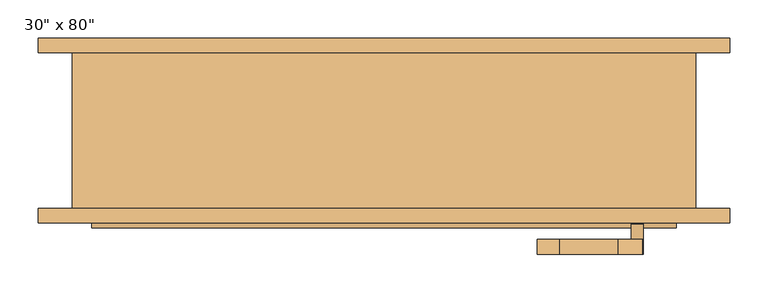
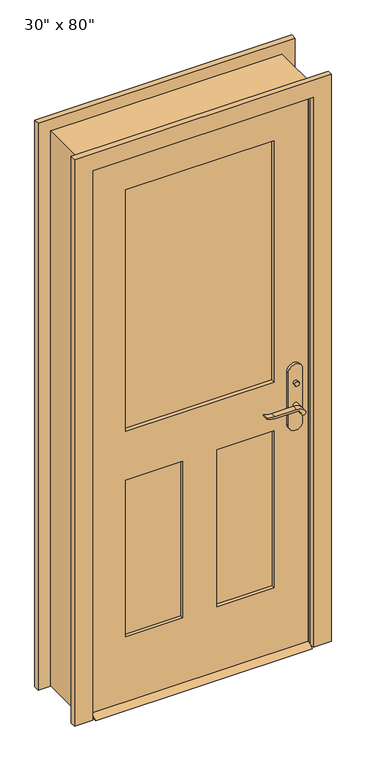
"""IFC4 building model written with IfcOpenShell, lengths in millimetres: door geometry."""

from ifc_helpers import new_model, si_unit, point, frame, frame_2d, origin, place, context, project, spatial, polyline, circle_curve, trimmed, segment, composite_curve, outline, extrude, faceted_brep, source, transform, mapped, element, save


def door_7e6851c9(model_context):
    return source(origin(), model_context, "Body", "SolidModel", [
        extrude(outline(polyline([(-63.5, 12.7), (-38.1, 0.0), (-123.825, 0.0), (-98.425, 12.7), (-63.5, 12.7)])), frame((-381.0, 0.0, 0.0), z_axis=(1.0, 0.0, 0.0), x_axis=(0.0, 1.0, 0.0)), (0.0, 0.0, 1.0), 762.0),
        extrude(outline(polyline([(335.2, -43.5), (335.2, -53.5), (325.2, -53.5), (325.2, -43.5), (335.2, -43.5)])), frame((0.0, 0.0, 981.9), z_axis=(0.0, 0.0, 1.0), x_axis=(1.0, 0.0, 0.0)), (0.0, 0.0, 1.0), 30.0),
        extrude(outline(composite_curve([segment(trimmed(circle_curve(frame_2d((996.9, 330.2)), 8.0), [point((996.9, 322.2))], [point((996.9, 338.2))], False, "CARTESIAN"), True, "CONTINUOUS"), segment(trimmed(circle_curve(frame_2d((996.9, 330.2)), 8.0), [point((996.9, 338.2))], [point((996.9, 322.2))], False, "CARTESIAN"), True, "CONTINUOUS")], self_intersect=False)), frame((0.0, -118.425, 0.0), z_axis=(0.0, 1.0, 0.0), x_axis=(0.0, 0.0, 1.0)), (0.0, 0.0, 1.0), 10.0),
        extrude(outline(composite_curve([segment(trimmed(circle_curve(frame_2d((897.1555521, 306.5324871)), 37.2832219), [point((919.0523287, 336.7081363))], [point((934.4, 304.8325667))], False, "CARTESIAN"), True, "CONTINUOUS"), segment(polyline([(934.4, 304.8325667), (934.4, 228.5564091)]), True, "CONTINUOUS"), segment(trimmed(circle_curve(frame_2d((1017.6850638, 228.6227909)), 83.2850902), [point((934.4, 228.5564091))], [point((939.4, 200.2))], True, "CARTESIAN"), True, "CONTINUOUS"), segment(polyline([(939.4, 200.2), (936.6135558, 200.2)]), True, "CONTINUOUS"), segment(trimmed(circle_curve(frame_2d((986.6709207, 232.1396612)), 59.3791355), [point((936.6135558, 200.2))], [point((927.4, 228.5564091))], False, "CARTESIAN"), True, "CONTINUOUS"), segment(polyline([(927.4, 228.5564091), (927.4, 304.8138099)]), True, "CONTINUOUS"), segment(trimmed(circle_curve(frame_2d((909.2738613, 304.8138099)), 18.1261387), [point((927.4, 304.8138099))], [point((914.4, 322.2))], True, "CARTESIAN"), True, "CONTINUOUS"), segment(trimmed(circle_curve(frame_2d((914.4, 330.2)), 8.0), [point((914.4, 322.2))], [point((919.0523287, 336.7081363))], False, "CARTESIAN"), True, "CONTINUOUS")], self_intersect=False)), frame((0.0, -23.5, 0.0), z_axis=(0.0, 1.0, 0.0), x_axis=(0.0, 0.0, 1.0)), (0.0, 0.0, 1.0), 20.0),
        extrude(outline(composite_curve([segment(trimmed(circle_curve(frame_2d((914.4, 330.2)), 8.0), [point((914.3999903, 322.2))], [point((919.0523287, 336.7081363))], False, "CARTESIAN"), True, "CONTINUOUS"), segment(trimmed(circle_curve(frame_2d((897.1555521, 306.5324871)), 37.2832219), [point((919.0523287, 336.7081363))], [point((934.4, 304.8325667))], False, "CARTESIAN"), True, "CONTINUOUS"), segment(polyline([(934.4, 304.8325667), (934.4, 228.5564091)]), True, "CONTINUOUS"), segment(trimmed(circle_curve(frame_2d((1017.6850638, 228.6227909)), 83.2850902), [point((934.4, 228.5564091))], [point((939.4, 200.2))], True, "CARTESIAN"), True, "CONTINUOUS"), segment(polyline([(939.4, 200.2), (936.6135558, 200.2)]), True, "CONTINUOUS"), segment(trimmed(circle_curve(frame_2d((986.6709207, 232.1396612)), 59.3791355), [point((936.6135558, 200.2))], [point((927.4, 228.5564091))], False, "CARTESIAN"), True, "CONTINUOUS"), segment(polyline([(927.4, 228.5564091), (927.4, 304.8138122)]), True, "CONTINUOUS"), segment(trimmed(circle_curve(frame_2d((909.2738682, 304.8138122)), 18.1261318), [point((927.4, 304.8138122))], [point((914.3999903, 322.2))], True, "CARTESIAN"), True, "CONTINUOUS")], self_intersect=False)), frame((0.0, -158.425, 0.0), z_axis=(0.0, 1.0, 0.0), x_axis=(0.0, 0.0, 1.0)), (0.0, 0.0, 1.0), 20.0),
        extrude(outline(composite_curve([segment(trimmed(circle_curve(frame_2d((914.4, 330.2)), 8.0), [point((914.4, 322.2))], [point((914.4, 338.2))], False, "CARTESIAN"), True, "CONTINUOUS"), segment(trimmed(circle_curve(frame_2d((914.4, 330.2)), 8.0), [point((914.4, 338.2))], [point((914.4, 322.2))], False, "CARTESIAN"), True, "CONTINUOUS")], self_intersect=False)), frame((0.0, -53.5, 0.0), z_axis=(0.0, 1.0, 0.0), x_axis=(0.0, 0.0, 1.0)), (0.0, 0.0, 1.0), 30.0),
        extrude(outline(composite_curve([segment(trimmed(circle_curve(frame_2d((914.4, 330.2)), 8.0), [point((914.4, 322.2))], [point((914.4, 338.2))], False, "CARTESIAN"), True, "CONTINUOUS"), segment(trimmed(circle_curve(frame_2d((914.4, 330.2)), 8.0), [point((914.4, 338.2))], [point((914.4, 322.2))], False, "CARTESIAN"), True, "CONTINUOUS")], self_intersect=False)), frame((0.0, -138.425, 0.0), z_axis=(0.0, 1.0, 0.0), x_axis=(0.0, 0.0, 1.0)), (0.0, 0.0, 1.0), 30.0),
        extrude(outline(composite_curve([segment(polyline([(844.4, 355.2), (1039.4, 355.2)]), True, "CONTINUOUS"), segment(trimmed(circle_curve(frame_2d((1039.4, 330.2)), 25.0), [point((1039.4, 355.2))], [point((1039.4, 305.2))], False, "CARTESIAN"), True, "CONTINUOUS"), segment(polyline([(1039.4, 305.2), (844.4, 305.2)]), True, "CONTINUOUS"), segment(trimmed(circle_curve(frame_2d((844.4, 330.2)), 25.0), [point((844.4, 305.2))], [point((844.4, 355.2))], False, "CARTESIAN"), True, "CONTINUOUS")], self_intersect=False)), frame((0.0, -63.5, 0.0), z_axis=(0.0, 1.0, 0.0), x_axis=(0.0, 0.0, 1.0)), (0.0, 0.0, 1.0), 10.0),
        extrude(outline(composite_curve([segment(polyline([(844.4, 355.2), (1039.4, 355.2)]), True, "CONTINUOUS"), segment(trimmed(circle_curve(frame_2d((1039.4, 330.2)), 25.0), [point((1039.4, 355.2))], [point((1039.4, 305.2))], False, "CARTESIAN"), True, "CONTINUOUS"), segment(polyline([(1039.4, 305.2), (844.4, 305.2)]), True, "CONTINUOUS"), segment(trimmed(circle_curve(frame_2d((844.4, 330.2)), 25.0), [point((844.4, 305.2))], [point((844.4, 355.2))], False, "CARTESIAN"), True, "CONTINUOUS")], self_intersect=False)), frame((0.0, -108.425, 0.0), z_axis=(0.0, 1.0, 0.0), x_axis=(0.0, 0.0, 1.0)), (0.0, 0.0, 1.0), 10.0),
        extrude(outline(polyline([(2032.0, -381.0), (12.7, -381.0), (12.7, 381.0), (2032.0, 381.0), (2032.0, -381.0)]), holes=[polyline([(1016.0, -260.35), (1911.35, -260.35), (1911.35, 260.35), (1016.0, 260.35), (1016.0, -260.35)]), polyline([(835.025, -60.325), (254.0, -60.325), (254.0, -260.35), (835.025, -260.35), (835.025, -60.325)]), polyline([(835.025, 260.35), (254.0, 260.35), (254.0, 60.325), (835.025, 60.325), (835.025, 260.35)])]), frame((0.0, -98.425, 0.0), z_axis=(0.0, 1.0, 0.0), x_axis=(0.0, 0.0, 1.0)), (0.0, 0.0, 1.0), 34.925),
        faceted_brep([(406.4, -98.425, 0.0), (381.0, -98.425, 0.0), (381.0, -63.5, 0.0), (368.3, -63.5, 0.0), (368.3, -28.575, 0.0), (381.0, -28.575, 0.0), (381.0, 104.775, 0.0), (406.4, 104.775, 0.0), (406.4, 104.775, 2057.4), (406.4, -98.425, 2057.4), (381.0, 104.775, 2032.0), (-381.0, 104.775, 2032.0), (-381.0, 104.775, 0.0), (-406.4, 104.775, 0.0), (-406.4, 104.775, 2057.4), (381.0, -28.575, 2032.0), (368.3, -28.575, 2019.3), (-368.3, -28.575, 2019.3), (-368.3, -28.575, 0.0), (-381.0, -28.575, 0.0), (-381.0, -28.575, 2032.0), (368.3, -63.5, 2019.3), (381.0, -63.5, 2032.0), (-381.0, -63.5, 2032.0), (-381.0, -63.5, 0.0), (-368.3, -63.5, 0.0), (-368.3, -63.5, 2019.3), (381.0, -98.425, 2032.0), (-406.4, -98.425, 2057.4), (-406.4, -98.425, 0.0), (-381.0, -98.425, 0.0), (-381.0, -98.425, 2032.0)], [[[0, 1, 2, 3, 4, 5, 6, 7]], [[7, 8, 9, 0]], [[6, 10, 11, 12, 13, 14, 8, 7]], [[5, 15, 10, 6]], [[4, 16, 17, 18, 19, 20, 15, 5]], [[3, 21, 16, 4]], [[2, 22, 23, 24, 25, 26, 21, 3]], [[1, 27, 22, 2]], [[0, 9, 28, 29, 30, 31, 27, 1]], [[8, 14, 28, 9]], [[15, 20, 11, 10]], [[21, 26, 17, 16]], [[27, 31, 23, 22]], [[29, 13, 12, 19, 18, 25, 24, 30]], [[14, 13, 29, 28]], [[20, 19, 12, 11]], [[26, 25, 18, 17]], [[31, 30, 24, 23]]]),
        extrude(outline(polyline([(-60.325, -75.1416667), (-60.325, -86.7833333), (-260.35, -86.7833333), (-260.35, -75.1416667), (-60.325, -75.1416667)])), frame((0.0, 0.0, 254.0), z_axis=(0.0, 0.0, 1.0), x_axis=(1.0, 0.0, 0.0)), (0.0, 0.0, 1.0), 581.025),
        extrude(outline(polyline([(260.35, -75.1416667), (260.35, -86.7833333), (60.325, -86.7833333), (60.325, -75.1416667), (260.35, -75.1416667)])), frame((0.0, 0.0, 254.0), z_axis=(0.0, 0.0, 1.0), x_axis=(1.0, 0.0, 0.0)), (0.0, 0.0, 1.0), 581.025),
        extrude(outline(polyline([(260.35, -77.47), (260.35, -84.455), (-260.35, -84.455), (-260.35, -77.47), (260.35, -77.47)])), frame((0.0, 0.0, 1016.0), z_axis=(0.0, 0.0, 1.0), x_axis=(1.0, 0.0, 0.0)), (0.0, 0.0, 1.0), 895.35),
        extrude(outline(polyline([(0.0, -387.35), (2038.35, -387.35), (2038.35, 387.35), (0.0, 387.35), (0.0, 450.85), (2101.85, 450.85), (2101.85, -450.85), (0.0, -450.85), (0.0, -387.35)])), frame((0.0, 104.775, 0.0), z_axis=(0.0, 1.0, 0.0), x_axis=(0.0, 0.0, 1.0)), (0.0, 0.0, 1.0), 19.05),
        extrude(outline(polyline([(0.0, -387.35), (2038.35, -387.35), (2038.35, 387.35), (0.0, 387.35), (0.0, 450.85), (2101.85, 450.85), (2101.85, -450.85), (0.0, -450.85), (0.0, -387.35)])), frame((0.0, -117.475, 0.0), z_axis=(0.0, 1.0, 0.0), x_axis=(0.0, 0.0, 1.0)), (0.0, 0.0, 1.0), 19.05),
    ])


if __name__ == "__main__":
    model = new_model("IFC4")
    model_context = context("Model", 3, world=origin())
    ifc_project = project(units=[si_unit("LENGTHUNIT", "METRE", prefix="MILLI")], contexts=[model_context])
    site = spatial("IfcSite", under=ifc_project)
    building = spatial("IfcBuilding", under=site)
    placement = place(None, origin())
    door_shape = door_7e6851c9(model_context)
    element("IfcDoor", 1, ObjectType="30\" x 80\"", at=placement, inside=building, context=model_context, shape_type="MappedRepresentation", body=[
        mapped(door_shape, transform((0.0, 0.0, 0.0), x_axis=(1.0, 0.0, 0.0), y_axis=(0.0, 1.0, 0.0), z_axis=(0.0, 0.0, 1.0))),
    ])
    save(model, "model.ifc")

# Revit data of these elements
# Type "30\" x 80\""
#   Type Mark = "9"
#   Assembly Code = "B2030100"
#   Analytic Construction = "French door, wood frame with single glass"
#   Top Rail = 0' - 4 3/4"
#   Threshold Offset [instance default] = 0' - 0 1/2"
#   Thickness = 0' - 1 3/8"
#   Thermal Resistance (R) = 1.0696 (h·ft²·°F)/BTU
#   Swing Angle [instance default] = 90.00°
#   Stiles = 0' - 4 3/4"
#   Rough Width = 2' - 8"
#   Rough Height = 6' - 9"
#   Lock Rail = 0' - 7 1/8"
#   Height = 6' - 8"
#   Width = 2' - 6"
#   Heat Transfer Coefficient (U) = 0.9350 BTU/(h·ft²·°F)
#   Door Offset [instance default] = 0' - 0"
#   Bottom Rail = 0' - 9 1/2"
#   Threshold [instance default] = yes
#   Function = 1
#   Exterior Trim [instance default] = yes
#   Trim Material = Cherry
#   Threshold Material = Cherry
#   Panel Material = Cherry
#   Glazing = Glass
#   Frame Material = Cherry
#   Door Handle Material = Aluminum
#   Visual Light Transmittance = 0
#   Solar Heat Gain Coefficient = 0
#   Wall Closure = (empty or 0)
#   Construction Type = (empty or 0)
# Element 1 (IfcDoor, "30\" x 80\"")
#   Materials on its faces: "Cherry", "Aluminum", "Glass"
# Materials
#   "Cherry": class "Wood", colour RGB 226 177 128, transparency 0, Description = "Prunus Serotina", Cost = 0
#   "Glass": class "Glass", colour RGB 0 128 192, transparency 0.75, Description = "Soda Lime Glass", Cost = 0
#   "Aluminum": class "Metal", colour RGB 247 247 247, transparency 0, Description = "Aluminum 6061", Cost = 0
